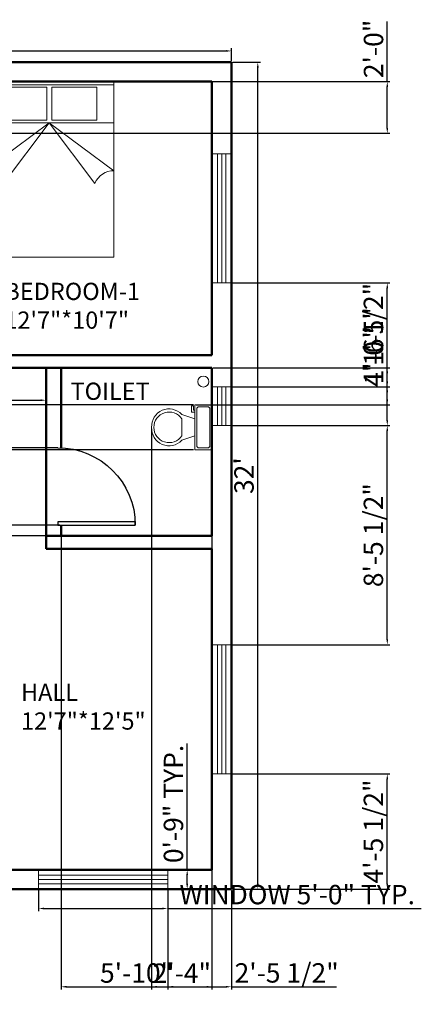
# Model space of a CAD drawing. Units: inches. Extents: x 2181 to 2717, y 1819 to 2296.
# Tile 5 of 5: x 2531 to 2717, y 1819 to 2276. Entities that reach past the tile are written whole.
import ezdxf

# ---------------------------------------------------------------- set-up
doc = ezdxf.new("R2010")
doc.units = ezdxf.units.IN
for name, color, linetype, lineweight in [('A-ANNO-DIMS', 2, 'Continuous', 13), ('A-AREA-IDEN', 7, 'Continuous', 25), ('A-DOOR', 3, 'Continuous', 25), ('A-FLOR-FIXT', 8, 'Continuous', 18), ('A-FURN', 8, 'Continuous', 18), ('A-GLAZ', 4, 'Continuous', 18), ('A-WALL', 7, 'Continuous', 50)]:
    doc.layers.add(name, color=color, linetype=linetype, lineweight=lineweight)
doc.styles.get("Standard").update_dxf_attribs({"font": 'arial.ttf'})
doc.dimstyles.new('ISO-25', dxfattribs={"dimtxt": 9, "dimasz": 2.5, "dimexe": 1.25, "dimexo": 0.625, "dimtad": 1, "dimlunit": 3, "dimtxsty": 'Standard', "dimcen": 2.5, "dimadec": 0, "dimazin": 0, "dimtfac": 1, "dimtmove": 0, "dimatfit": 3, "dimfxl": 1, "dimarcsym": 0})

# ---------------------------------------------------------------- blocks, each defined once
blk = doc.blocks.new('*U4')
for p, q in [((9.5, -6), (9.5, -2)), ((-10, -8.5), (-8, -8.5)), ((-10, -9.5), (-10, -8.5)), ((-8, -8.5), (-8, -8)), ((-7, -8), (-7, -9.5)), ((-4, -8), (-6, -14)), ((4, -8), (6, -14)), ((-7, -9.5), (-10, -9.5)), ((4, -14), (-4, -14))]:
    blk.add_line(p, q)
blk.add_lwpolyline([(10.5, -8), (10.5, 0), (-10.5, 0), (-10.5, -8)], close=True)
for points in [[(-9.5, -2), (-9.5, -6)], [(8.5, -1), (-8.5, -1)], [(-8.5, -7), (8.5, -7)]]:
    blk.add_lwpolyline(points)
for centre, radius, start, end in [((-8.625, -1.875), 0.8839, 81.8699, 188.1301), ((8.625, -1.875), 0.8839, 351.8699, 98.1301), ((-8.625, -6.125), 0.8839, 171.869898, 278.1301), ((8.625, -6.125), 0.8839, 261.8699, 8.1301), ((-0.4772, -19.9188), 8.0953, 133.01722, 273.38), ((0.0374, -19.8731), 7.127, 124.50543, 269.7), ((-0.0373, -19.8731), 7.127, 270.3, 55.4946), ((0.4773, -19.9188), 8.0953, 266.62, 46.9828)]:
    blk.add_arc(centre, radius, start, end)
blk = doc.blocks.new('*U2')
for p, q in [((0, 0), (0, -6)), ((40, 0), (40, -6))]:
    blk.add_line(p, q)
blk.add_lwpolyline([(0, 0), (0, 40), (1.75, 40), (1.75, 0)], close=True)
blk.add_arc((0, 0), 40, 0, 90)
blk = doc.blocks.new('*D8')
at = {"layer": 'A-ANNO-DIMS', "color": 0, "lineweight": -2, "transparency": 16777216}
for p, q in [((2329.35, 2256.83), (2329.35, 2262.67)), ((2331.85, 2261.42), (2626.85, 2261.42)), ((2629.35, 2256.83), (2629.35, 2262.67))]:
    blk.add_line(p, q, dxfattribs=at)
at = {"layer": 'A-ANNO-DIMS', "color": 0, "transparency": 16777216}
for points in [[(2331.85, 2261.84), (2331.85, 2261.01), (2329.35, 2261.42)], [(2626.85, 2261.84), (2626.85, 2261.01), (2629.35, 2261.42)]]:
    blk.add_solid(points, dxfattribs=at)
at = {"layer": 'Defpoints', "color": 0, "transparency": 16777216}
for p in [(2629.35, 2261.42), (2329.35, 2256.2), (2629.35, 2256.2)]:
    blk.add_point(p, dxfattribs=at)
at = {"layer": 'A-ANNO-DIMS', "color": 0, "transparency": 16777216, "insert": (2479.35, 2266.64), "char_height": 9, "attachment_point": 5}
blk.add_mtext("25'", dxfattribs=at)
blk = doc.blocks.new('*D9')
at = {"layer": 'A-ANNO-DIMS', "color": 0, "lineweight": -2, "transparency": 16777216}
for p, q in [((2629.97, 2256.2), (2642.85, 2256.2)), ((2641.6, 1874.7), (2641.6, 2253.7)), ((2629.97, 1872.2), (2642.85, 1872.2))]:
    blk.add_line(p, q, dxfattribs=at)
at = {"layer": 'A-ANNO-DIMS', "color": 0, "transparency": 16777216}
for points in [[(2641.19, 2253.7), (2642.02, 2253.7), (2641.6, 2256.2)], [(2641.19, 1874.7), (2642.02, 1874.7), (2641.6, 1872.2)]]:
    blk.add_solid(points, dxfattribs=at)
at = {"layer": 'Defpoints', "color": 0, "transparency": 16777216}
for p in [(2629.35, 2256.2), (2641.6, 2256.2), (2629.35, 1872.2)]:
    blk.add_point(p, dxfattribs=at)
at = {"layer": 'A-ANNO-DIMS', "color": 0, "transparency": 16777216, "insert": (2636.38, 2064.2), "char_height": 9, "attachment_point": 5, "rotation": 90}
blk.add_mtext("32'", dxfattribs=at)
blk = doc.blocks.new('*D13')
at = {"layer": 'A-ANNO-DIMS', "color": 0, "lineweight": -2, "transparency": 16777216}
for p, q in [((2445.35, 2113.58), (2445.35, 2097.98)), ((2543.35, 2113.58), (2543.35, 2097.98)), ((2447.85, 2099.23), (2540.85, 2099.23))]:
    blk.add_line(p, q, dxfattribs=at)
at = {"layer": 'A-ANNO-DIMS', "color": 0, "transparency": 16777216}
for points in [[(2447.85, 2099.65), (2447.85, 2098.81), (2445.35, 2099.23)], [(2540.85, 2099.65), (2540.85, 2098.81), (2543.35, 2099.23)]]:
    blk.add_solid(points, dxfattribs=at)
at = {"layer": 'Defpoints', "color": 0, "transparency": 16777216}
for p in [(2445.35, 2114.2), (2543.35, 2114.2), (2543.35, 2099.23)]:
    blk.add_point(p, dxfattribs=at)
at = {"layer": 'A-ANNO-DIMS', "color": 0, "transparency": 16777216, "insert": (2494.35, 2104.45), "char_height": 9, "attachment_point": 5}
blk.add_mtext('8\'-2"', dxfattribs=at)
blk = doc.blocks.new('WIN-60IN')
for p, q in [((0, 0), (0, 9)), ((60, 6.5), (0, 6.5)), ((60, 0), (60, 9)), ((60, 4.5), (0, 4.5)), ((60, 2.5), (0, 2.5))]:
    blk.add_line(p, q)
blk = doc.blocks.new('BED-QUEEN-PLAN')
for p, q in [((60.01, 81.47), (0, 81.47)), ((0, 81.47), (0, 80)), ((0.01, 0), (0.01, 80)), ((0.01, 80), (60.01, 80)), ((8.01, 78.8), (28.81, 78.8)), ((8.01, 63.6), (8.01, 78.8)), ((28.81, 78.8), (28.81, 63.6)), ((31.21, 78.8), (52.01, 78.8)), ((31.21, 63.6), (31.21, 78.8)), ((52.01, 78.8), (52.01, 63.6)), ((60.01, 80), (60.01, 81.47)), ((60.01, 80), (60.01, 0)), ((60.01, 62.35), (0.01, 62.35)), ((30.01, 62.35), (0.01, 40)), ((28.81, 63.6), (8.01, 63.6)), ((8.81, 34.19), (30.01, 62.35)), ((30.01, 62.35), (60.01, 40)), ((51.22, 34.19), (30.01, 62.35)), ((52.01, 63.6), (31.21, 63.6)), ((60.01, 0), (0.01, 0))]:
    blk.add_line(p, q)
for centre, start, end in [((0.34, 30.93), 21.0875, 92.0428), ((59.69, 30.93), 87.9572, 158.9125)]:
    blk.add_arc(centre, 9.08, start, end)
blk = doc.blocks.new('*D17')
at = {"layer": 'A-ANNO-DIMS', "color": 0, "lineweight": -2, "transparency": 16777216}
for p, q in [((2539.85, 1871.58), (2539.85, 1861.95)), ((2599.85, 1871.58), (2599.85, 1861.95)), ((2542.35, 1863.2), (2597.35, 1863.2)), ((2599.85, 1863.2), (2717.48, 1863.2))]:
    blk.add_line(p, q, dxfattribs=at)
at = {"layer": 'A-ANNO-DIMS', "color": 0, "transparency": 16777216}
for points in [[(2542.35, 1863.62), (2542.35, 1862.79), (2539.85, 1863.2)], [(2597.35, 1863.62), (2597.35, 1862.79), (2599.85, 1863.2)]]:
    blk.add_solid(points, dxfattribs=at)
at = {"layer": 'Defpoints', "color": 0, "transparency": 16777216}
for p in [(2539.85, 1872.2), (2599.85, 1872.2), (2599.85, 1863.2)]:
    blk.add_point(p, dxfattribs=at)
at = {"layer": 'A-ANNO-DIMS', "color": 0, "transparency": 16777216, "insert": (2659.92, 1868.49), "char_height": 9, "attachment_point": 5}
blk.add_mtext('WINDOW 5\'-0" TYP.', dxfattribs=at)
blk = doc.blocks.new('*D18')
at = {"layer": 'A-ANNO-DIMS', "color": 0, "lineweight": -2, "transparency": 16777216}
for p, q in [((2608.85, 1881.2), (2608.85, 1939.81)), ((2600.47, 1881.2), (2610.1, 1881.2)), ((2608.85, 1874.7), (2608.85, 1878.7)), ((2600.47, 1872.2), (2610.1, 1872.2))]:
    blk.add_line(p, q, dxfattribs=at)
at = {"layer": 'A-ANNO-DIMS', "color": 0, "transparency": 16777216}
for points in [[(2608.43, 1878.7), (2609.26, 1878.7), (2608.85, 1881.2)], [(2608.43, 1874.7), (2609.26, 1874.7), (2608.85, 1872.2)]]:
    blk.add_solid(points, dxfattribs=at)
at = {"layer": 'Defpoints', "color": 0, "transparency": 16777216}
for p in [(2599.85, 1881.2), (2608.85, 1881.2), (2599.85, 1872.2)]:
    blk.add_point(p, dxfattribs=at)
at = {"layer": 'A-ANNO-DIMS', "color": 0, "transparency": 16777216, "insert": (2603.63, 1911.76), "char_height": 9, "attachment_point": 5, "rotation": 90}
blk.add_mtext('0\'-9" TYP.', dxfattribs=at)
blk = doc.blocks.new('*D29')
at = {"layer": 'A-ANNO-DIMS', "color": 0, "lineweight": -2, "transparency": 16777216}
for p, q in [((2701.7, 2105.45), (2701.7, 2132.28)), ((2629.97, 2105.45), (2702.95, 2105.45)), ((2701.7, 2089.95), (2701.7, 2102.95)), ((2629.97, 2087.45), (2702.95, 2087.45))]:
    blk.add_line(p, q, dxfattribs=at)
at = {"layer": 'A-ANNO-DIMS', "color": 0, "transparency": 16777216}
for points in [[(2701.28, 2102.95), (2702.11, 2102.95), (2701.7, 2105.45)], [(2701.28, 2089.95), (2702.11, 2089.95), (2701.7, 2087.45)]]:
    blk.add_solid(points, dxfattribs=at)
at = {"layer": 'Defpoints', "color": 0, "transparency": 16777216}
for p in [(2629.35, 2105.45), (2701.7, 2105.45), (2629.35, 2087.45)]:
    blk.add_point(p, dxfattribs=at)
at = {"layer": 'A-ANNO-DIMS', "color": 0, "transparency": 16777216, "insert": (2696.48, 2120.11), "char_height": 9, "attachment_point": 5, "rotation": 90}
blk.add_mtext('1\'-6"', dxfattribs=at)
blk = doc.blocks.new('*D30')
at = {"layer": 'A-ANNO-DIMS', "color": 0, "lineweight": -2, "transparency": 16777216}
for p, q in [((2629.97, 2087.45), (2702.95, 2087.45)), ((2701.7, 1988.2), (2701.7, 2084.95)), ((2629.97, 1985.7), (2702.95, 1985.7))]:
    blk.add_line(p, q, dxfattribs=at)
at = {"layer": 'A-ANNO-DIMS', "color": 0, "transparency": 16777216}
for points in [[(2701.28, 2084.95), (2702.11, 2084.95), (2701.7, 2087.45)], [(2701.28, 1988.2), (2702.11, 1988.2), (2701.7, 1985.7)]]:
    blk.add_solid(points, dxfattribs=at)
at = {"layer": 'Defpoints', "color": 0, "transparency": 16777216}
for p in [(2629.35, 2087.45), (2701.7, 2087.45), (2629.35, 1985.7)]:
    blk.add_point(p, dxfattribs=at)
at = {"layer": 'A-ANNO-DIMS', "color": 0, "transparency": 16777216, "insert": (2696.42, 2036.58), "char_height": 9, "attachment_point": 5, "rotation": 90}
blk.add_mtext('8\'-5 1/2"', dxfattribs=at)
blk = doc.blocks.new('*D31')
at = {"layer": 'A-ANNO-DIMS', "color": 0, "lineweight": -2, "transparency": 16777216}
for p, q in [((2629.97, 2153.7), (2702.95, 2153.7)), ((2701.7, 2107.95), (2701.7, 2151.2)), ((2629.97, 2105.45), (2702.95, 2105.45))]:
    blk.add_line(p, q, dxfattribs=at)
at = {"layer": 'A-ANNO-DIMS', "color": 0, "transparency": 16777216}
for points in [[(2701.28, 2151.2), (2702.11, 2151.2), (2701.7, 2153.7)], [(2701.28, 2107.95), (2702.11, 2107.95), (2701.7, 2105.45)]]:
    blk.add_solid(points, dxfattribs=at)
at = {"layer": 'Defpoints', "color": 0, "transparency": 16777216}
for p in [(2629.35, 2153.7), (2701.7, 2153.7), (2629.35, 2105.45)]:
    blk.add_point(p, dxfattribs=at)
at = {"layer": 'A-ANNO-DIMS', "color": 0, "transparency": 16777216, "insert": (2696.42, 2129.58), "char_height": 9, "attachment_point": 5, "rotation": 90}
blk.add_mtext('4\'-0 1/2"', dxfattribs=at)
blk = doc.blocks.new('*D32')
at = {"layer": 'A-ANNO-DIMS', "color": 0, "lineweight": -2, "transparency": 16777216}
for p, q in [((2629.97, 1925.7), (2702.95, 1925.7)), ((2701.7, 1874.7), (2701.7, 1923.2)), ((2629.97, 1872.2), (2702.95, 1872.2))]:
    blk.add_line(p, q, dxfattribs=at)
at = {"layer": 'A-ANNO-DIMS', "color": 0, "transparency": 16777216}
for points in [[(2701.28, 1923.2), (2702.11, 1923.2), (2701.7, 1925.7)], [(2701.28, 1874.7), (2702.11, 1874.7), (2701.7, 1872.2)]]:
    blk.add_solid(points, dxfattribs=at)
at = {"layer": 'Defpoints', "color": 0, "transparency": 16777216}
for p in [(2629.35, 1925.7), (2701.7, 1925.7), (2629.35, 1872.2)]:
    blk.add_point(p, dxfattribs=at)
at = {"layer": 'A-ANNO-DIMS', "color": 0, "transparency": 16777216, "insert": (2696.42, 1898.95), "char_height": 9, "attachment_point": 5, "rotation": 90}
blk.add_mtext('4\'-5 1/2"', dxfattribs=at)
blk = doc.blocks.new('*D33')
at = {"layer": 'A-ANNO-DIMS', "color": 0, "lineweight": -2, "transparency": 16777216}
for p, q in [((2599.85, 1871.58), (2599.85, 1825.6)), ((2629.35, 1871.58), (2629.35, 1825.6)), ((2602.35, 1826.85), (2626.85, 1826.85)), ((2629.35, 1826.85), (2678.15, 1826.85))]:
    blk.add_line(p, q, dxfattribs=at)
at = {"layer": 'A-ANNO-DIMS', "color": 0, "transparency": 16777216}
for points in [[(2602.35, 1827.27), (2602.35, 1826.44), (2599.85, 1826.85)], [(2626.85, 1827.27), (2626.85, 1826.44), (2629.35, 1826.85)]]:
    blk.add_solid(points, dxfattribs=at)
at = {"layer": 'Defpoints', "color": 0, "transparency": 16777216}
for p in [(2599.85, 1872.2), (2629.35, 1872.2), (2629.35, 1826.85)]:
    blk.add_point(p, dxfattribs=at)
at = {"layer": 'A-ANNO-DIMS', "color": 0, "transparency": 16777216, "insert": (2655, 1832.13), "char_height": 9, "attachment_point": 5}
blk.add_mtext('2\'-5 1/2"', dxfattribs=at)
blk = doc.blocks.new('*D39')
at = {"layer": 'A-ANNO-DIMS', "color": 0, "lineweight": -2, "transparency": 16777216}
for p, q in [((2550.35, 2035.58), (2550.35, 1825.6)), ((2620.35, 2035.58), (2620.35, 1825.6)), ((2552.85, 1826.85), (2617.85, 1826.85))]:
    blk.add_line(p, q, dxfattribs=at)
at = {"layer": 'A-ANNO-DIMS', "color": 0, "transparency": 16777216}
for points in [[(2552.85, 1827.27), (2552.85, 1826.44), (2550.35, 1826.85)], [(2617.85, 1827.27), (2617.85, 1826.44), (2620.35, 1826.85)]]:
    blk.add_solid(points, dxfattribs=at)
at = {"layer": 'Defpoints', "color": 0, "transparency": 16777216}
for p in [(2550.35, 2036.2), (2620.35, 2036.2), (2620.35, 1826.85)]:
    blk.add_point(p, dxfattribs=at)
at = {"layer": 'A-ANNO-DIMS', "color": 0, "transparency": 16777216, "insert": (2585.35, 1832.07), "char_height": 9, "attachment_point": 5}
blk.add_mtext('5\'-10"', dxfattribs=at)
blk = doc.blocks.new('*D42')
at = {"layer": 'A-ANNO-DIMS', "color": 0, "lineweight": -2, "transparency": 16777216}
for p, q in [((2701.7, 2247.2), (2701.7, 2275.03)), ((2462.97, 2247.2), (2702.95, 2247.2)), ((2701.7, 2225.7), (2701.7, 2244.7)), ((2462.97, 2223.2), (2702.95, 2223.2))]:
    blk.add_line(p, q, dxfattribs=at)
at = {"layer": 'A-ANNO-DIMS', "color": 0, "transparency": 16777216}
for points in [[(2701.28, 2244.7), (2702.11, 2244.7), (2701.7, 2247.2)], [(2701.28, 2225.7), (2702.11, 2225.7), (2701.7, 2223.2)]]:
    blk.add_solid(points, dxfattribs=at)
at = {"layer": 'Defpoints', "color": 0, "transparency": 16777216}
for p in [(2462.35, 2247.2), (2701.7, 2247.2), (2462.35, 2223.2)]:
    blk.add_point(p, dxfattribs=at)
at = {"layer": 'A-ANNO-DIMS', "color": 0, "transparency": 16777216, "insert": (2696.48, 2262.37), "char_height": 9, "attachment_point": 5, "rotation": 90}
blk.add_mtext('2\'-0"', dxfattribs=at)
blk = doc.blocks.new('*D49')
at = {"layer": 'A-ANNO-DIMS', "color": 0, "lineweight": -2, "transparency": 16777216}
for p, q in [((2701.7, 2114.2), (2701.7, 2141.03)), ((2620.97, 2114.2), (2702.95, 2114.2)), ((2701.7, 2099.63), (2701.7, 2111.7)), ((2612.97, 2097.13), (2702.95, 2097.13))]:
    blk.add_line(p, q, dxfattribs=at)
at = {"layer": 'A-ANNO-DIMS', "color": 0, "transparency": 16777216}
for points in [[(2701.28, 2111.7), (2702.11, 2111.7), (2701.7, 2114.2)], [(2701.28, 2099.63), (2702.11, 2099.63), (2701.7, 2097.13)]]:
    blk.add_solid(points, dxfattribs=at)
at = {"layer": 'Defpoints', "color": 0, "transparency": 16777216}
for p in [(2620.35, 2114.2), (2701.7, 2114.2), (2612.35, 2097.13)]:
    blk.add_point(p, dxfattribs=at)
at = {"layer": 'A-ANNO-DIMS', "color": 0, "transparency": 16777216, "insert": (2696.48, 2128.87), "char_height": 9, "attachment_point": 5, "rotation": 90}
blk.add_mtext('1\'-5"', dxfattribs=at)
blk = doc.blocks.new('*D50')
at = {"layer": 'A-ANNO-DIMS', "color": 0, "lineweight": -2, "transparency": 16777216}
for p, q in [((2308, 2097.13), (2308, 2123.96)), ((2611.72, 2097.13), (2306.75, 2097.13)), ((2308, 2078.63), (2308, 2094.63)), ((2611.72, 2076.13), (2306.75, 2076.13))]:
    blk.add_line(p, q, dxfattribs=at)
at = {"layer": 'A-ANNO-DIMS', "color": 0, "transparency": 16777216}
for points in [[(2307.58, 2094.63), (2308.41, 2094.63), (2308, 2097.13)], [(2307.58, 2078.63), (2308.41, 2078.63), (2308, 2076.13)]]:
    blk.add_solid(points, dxfattribs=at)
at = {"layer": 'Defpoints', "color": 0, "transparency": 16777216}
for p in [(2308, 2097.13), (2612.35, 2097.13), (2612.35, 2076.13)]:
    blk.add_point(p, dxfattribs=at)
at = {"layer": 'A-ANNO-DIMS', "color": 0, "transparency": 16777216, "insert": (2302.78, 2111.79), "char_height": 9, "attachment_point": 5, "rotation": 90}
blk.add_mtext('1\'-9"', dxfattribs=at)
blk = doc.blocks.new('*D51')
at = {"layer": 'A-ANNO-DIMS', "color": 0, "lineweight": -2, "transparency": 16777216}
for p, q in [((2592.35, 2086), (2592.35, 1825.6)), ((2620.35, 2075.5), (2620.35, 1825.6)), ((2594.85, 1826.85), (2617.85, 1826.85))]:
    blk.add_line(p, q, dxfattribs=at)
at = {"layer": 'A-ANNO-DIMS', "color": 0, "transparency": 16777216}
for points in [[(2594.85, 1827.27), (2594.85, 1826.44), (2592.35, 1826.85)], [(2617.85, 1827.27), (2617.85, 1826.44), (2620.35, 1826.85)]]:
    blk.add_solid(points, dxfattribs=at)
at = {"layer": 'Defpoints', "color": 0, "transparency": 16777216}
for p in [(2592.35, 2086.63), (2620.35, 2076.13), (2620.35, 1826.85)]:
    blk.add_point(p, dxfattribs=at)
at = {"layer": 'A-ANNO-DIMS', "color": 0, "transparency": 16777216, "insert": (2606.35, 1832), "char_height": 9, "attachment_point": 5}
blk.add_mtext('2\'-4"', dxfattribs=at)
blk = doc.blocks.new('*D52')
at = {"layer": 'A-ANNO-DIMS', "color": 0, "lineweight": -2, "transparency": 16777216}
for p, q in [((2542.72, 2077.19), (2306.75, 2077.19)), ((2308, 2043.69), (2308, 2074.69)), ((2542.72, 2041.19), (2306.75, 2041.19))]:
    blk.add_line(p, q, dxfattribs=at)
at = {"layer": 'A-ANNO-DIMS', "color": 0, "transparency": 16777216}
for points in [[(2307.58, 2074.69), (2308.41, 2074.69), (2308, 2077.19)], [(2307.58, 2043.69), (2308.41, 2043.69), (2308, 2041.19)]]:
    blk.add_solid(points, dxfattribs=at)
at = {"layer": 'Defpoints', "color": 0, "transparency": 16777216}
for p in [(2308, 2077.19), (2543.35, 2077.19), (2543.35, 2041.19)]:
    blk.add_point(p, dxfattribs=at)
at = {"layer": 'A-ANNO-DIMS', "color": 0, "transparency": 16777216, "insert": (2302.77, 2059.19), "char_height": 9, "attachment_point": 5, "rotation": 90}
blk.add_mtext('3\'-0"', dxfattribs=at)
blk = doc.blocks.new('*D53')
at = {"layer": 'A-ANNO-DIMS', "color": 0, "lineweight": -2, "transparency": 16777216}
for p, q in [((2308, 2043.69), (2308, 2046.19)), ((2549.72, 2041.19), (2306.75, 2041.19)), ((2308, 2041.19), (2308, 2036.2)), ((2549.72, 2036.2), (2306.75, 2036.2)), ((2308, 2033.7), (2308, 2006.03))]:
    blk.add_line(p, q, dxfattribs=at)
at = {"layer": 'A-ANNO-DIMS', "color": 0, "transparency": 16777216}
for points in [[(2307.58, 2043.69), (2308.41, 2043.69), (2308, 2041.19)], [(2307.58, 2033.7), (2308.41, 2033.7), (2308, 2036.2)]]:
    blk.add_solid(points, dxfattribs=at)
at = {"layer": 'Defpoints', "color": 0, "transparency": 16777216}
for p in [(2550.35, 2041.19), (2308, 2036.2), (2550.35, 2036.2)]:
    blk.add_point(p, dxfattribs=at)
at = {"layer": 'A-ANNO-DIMS', "color": 0, "transparency": 16777216, "insert": (2302.78, 2018.62), "char_height": 9, "attachment_point": 5, "rotation": 90}
blk.add_mtext('0\'-5"', dxfattribs=at)
blk = doc.blocks.new('*D56')
at = {"layer": 'A-ANNO-DIMS', "color": 0, "lineweight": -2, "transparency": 16777216}
for p, q in [((2549.72, 2114.2), (2306.75, 2114.2)), ((2308, 2038.7), (2308, 2111.7)), ((2549.72, 2036.2), (2306.75, 2036.2))]:
    blk.add_line(p, q, dxfattribs=at)
at = {"layer": 'A-ANNO-DIMS', "color": 0, "transparency": 16777216}
for points in [[(2307.58, 2111.7), (2308.41, 2111.7), (2308, 2114.2)], [(2307.58, 2038.7), (2308.41, 2038.7), (2308, 2036.2)]]:
    blk.add_solid(points, dxfattribs=at)
at = {"layer": 'Defpoints', "color": 0, "transparency": 16777216}
for p in [(2308, 2114.2), (2550.35, 2114.2), (2550.35, 2036.2)]:
    blk.add_point(p, dxfattribs=at)
at = {"layer": 'A-ANNO-DIMS', "color": 0, "transparency": 16777216, "insert": (2302.78, 2075.2), "char_height": 9, "attachment_point": 5, "rotation": 90}
blk.add_mtext('6\'-6"', dxfattribs=at)

msp = doc.modelspace()

# ---------------------------------------------------------------- linework, layer by layer
at = {"layer": 'A-FLOR-FIXT'}
msp.add_circle((2616.346, 2107.897), 2.575, dxfattribs=at)
at = {"layer": 'A-GLAZ'}
for p, q in [((2620.346, 2105.45), (2629.346, 2105.45)), ((2622.846, 2105.45), (2622.846, 2087.45)), ((2624.846, 2105.45), (2624.846, 2087.45)), ((2626.846, 2105.45), (2626.846, 2087.45)), ((2620.346, 2087.45), (2629.346, 2087.45))]:
    msp.add_line(p, q, dxfattribs=at)
at = {"layer": 'A-WALL'}
for p, q in [((2329.346, 2256.205), (2629.346, 2256.205)), ((2629.346, 2256.205), (2629.346, 1872.205)), ((2469.346, 2247.205), (2620.346, 2247.205)), ((2620.346, 2247.205), (2620.346, 2120.205)), ((2510.745, 2120.205), (2620.346, 2120.205)), ((2338.346, 2114.205), (2620.346, 2114.205)), ((2543.346, 2114.205), (2543.346, 2030.205)), ((2550.346, 2114.205), (2550.346, 2077.152)), ((2620.346, 2114.205), (2620.346, 2036.205)), ((2550.346, 2041.187), (2550.346, 2036.205)), ((2543.346, 2036.205), (2620.346, 2036.205)), ((2543.346, 2030.205), (2620.346, 2030.205)), ((2620.346, 2030.205), (2620.346, 1881.205)), ((2519.346, 1881.205), (2620.346, 1881.205)), ((2329.346, 1872.205), (2629.346, 1872.205))]:
    msp.add_line(p, q, dxfattribs=at)

# ---------------------------------------------------------------- block references
at = {"layer": 'A-DOOR', "xscale": -0.9, "yscale": 0.9, "zscale": 0.9, "rotation": 270}
msp.add_blockref('*U2', (2548.746, 2041.187), dxfattribs=at)
at = {"layer": 'A-FLOR-FIXT', "rotation": 270.0000000000003}
msp.add_blockref('*U4', (2620.346, 2086.628), dxfattribs=at)
at = {"layer": 'A-FURN'}
msp.add_blockref('BED-QUEEN-PLAN', (2514.834, 2165.732), dxfattribs=at)
at = {"layer": 'A-GLAZ'}
for p, rotation in [((2620.347, 2213.705), 270.0000000000003), ((2620.347, 1985.705), 269.9999999999999)]:
    msp.add_blockref('WIN-60IN', p, dxfattribs=dict(at, rotation=rotation))
msp.add_blockref('WIN-60IN', (2539.846, 1872.205), dxfattribs=at)

# ---------------------------------------------------------------- texts
at = {"layer": 'A-AREA-IDEN', "char_height": 8, "attachment_point": 1}
for s, width, insert in [('BEDROOM-1\\P12\'7"*10\'7"', 37.99236, (2523.994, 2153.766)), ('TOILET', 27.2831, (2554.717, 2107.388)), ('HALL\\P12\'7"*12\'5"', 52.01638, (2531.721, 1967.594))]:
    msp.add_mtext_dynamic_manual_height_columns(s, width=width, gutter_width=12.5, heights=[0], dxfattribs=dict(at, insert=insert))

# ---------------------------------------------------------------- dimensions: what is measured, and where the dimension line sits
at = {"layer": 'A-ANNO-DIMS'}
dim = msp.add_linear_dim(base=(2629.346, 2261.425), p1=(2329.346, 2256.205), p2=(2629.346, 2256.205), dimstyle='ISO-25', override={"dimclrd": 0, "dimclre": 0, "dimclrt": 0}, dxfattribs=at)
dim.commit()
dim.dimension.update_dxf_attribs({"geometry": '*D8', "text_midpoint": (2479.346, 2261.425), "dimtype": 160})
for base, p1, p2, override, picture, middle in [((2701.696, 2247.205), (2462.346, 2223.205), (2462.346, 2247.205), {"dimdec": 1, "dimlfac": 1, "dimrnd": 0, "dimzin": 1, "dimdsep": 46, "dimlunit": 4, "dimfrac": 2}, '*D42', (2696.476, 2262.368)), ((2641.604, 2256.205), (2629.346, 1872.205), (2629.346, 2256.205), {"dimclrd": 0, "dimclre": 0, "dimclrt": 0}, '*D9', (2636.381, 2064.205)), ((2701.696, 2153.705), (2629.346, 2105.45), (2629.346, 2153.705), {"dimdec": 1, "dimlfac": 1, "dimrnd": 0, "dimzin": 1, "dimdsep": 46, "dimlunit": 4, "dimfrac": 2}, '*D31', (2696.418, 2129.577)), ((2701.696, 2114.205), (2612.346, 2097.128), (2620.346, 2114.205), {"dimdec": 1, "dimlfac": 1, "dimrnd": 0, "dimzin": 1, "dimdsep": 46, "dimlunit": 4, "dimfrac": 2}, '*D49', (2696.476, 2128.868)), ((2701.696, 2105.45), (2629.346, 2087.45), (2629.346, 2105.45), {"dimdec": 1, "dimlfac": 1, "dimrnd": 0, "dimzin": 1, "dimdsep": 46, "dimlunit": 4, "dimfrac": 2}, '*D29', (2696.476, 2120.113)), ((2307.996, 2097.128), (2612.346, 2076.128), (2612.346, 2097.128), {"dimdec": 1, "dimlfac": 1, "dimrnd": 0, "dimzin": 1, "dimdsep": 46, "dimlunit": 4, "dimfrac": 2}, '*D50', (2302.776, 2111.792)), ((2307.996, 2114.205), (2550.346, 2036.205), (2550.346, 2114.205), {"dimdec": 1, "dimlfac": 1, "dimrnd": 0, "dimzin": 1, "dimdsep": 46, "dimlunit": 4, "dimfrac": 2}, '*D56', (2302.776, 2075.205)), ((2701.696, 2087.45), (2629.346, 1985.705), (2629.346, 2087.45), {"dimdec": 1, "dimlfac": 1, "dimrnd": 0, "dimzin": 1, "dimdsep": 46, "dimlunit": 4, "dimfrac": 2}, '*D30', (2696.418, 2036.577)), ((2307.996, 2077.187), (2543.346, 2041.187), (2543.346, 2077.187), {"dimdec": 1, "dimlfac": 1, "dimrnd": 0, "dimzin": 1, "dimdsep": 46, "dimlunit": 4, "dimfrac": 2}, '*D52', (2302.773, 2059.187)), ((2307.996, 2036.205), (2550.346, 2041.187), (2550.346, 2036.205), {"dimdec": 1, "dimlfac": 1, "dimrnd": 0, "dimzin": 1, "dimdsep": 46, "dimlunit": 4, "dimfrac": 2}, '*D53', (2302.776, 2018.617)), ((2701.696, 1925.705), (2629.346, 1872.205), (2629.346, 1925.705), {"dimdec": 1, "dimlfac": 1, "dimrnd": 0, "dimzin": 1, "dimdsep": 46, "dimlunit": 4, "dimfrac": 2}, '*D32', (2696.418, 1898.955))]:
    dim = msp.add_linear_dim(base=base, p1=p1, p2=p2, angle=90, dimstyle='ISO-25', override=override, dxfattribs=at)
    dim.commit()
    dim.dimension.update_dxf_attribs({"geometry": picture, "text_midpoint": middle})
for base, p1, p2, override, picture, middle in [((2543.346, 2099.229), (2445.346, 2114.205), (2543.346, 2114.205), {"dimclrd": 0, "dimclre": 0, "dimclrt": 0}, '*D13', (2494.346, 2104.449)), ((2620.346, 1826.855), (2592.346, 2086.628), (2620.346, 2076.128), {"dimdec": 1, "dimlfac": 1, "dimrnd": 0, "dimzin": 1, "dimdsep": 46, "dimlunit": 4, "dimfrac": 2}, '*D51', (2606.346, 1831.998)), ((2620.346, 1826.855), (2550.346, 2036.205), (2620.346, 2036.205), {"dimdec": 1, "dimlfac": 1, "dimrnd": 0, "dimzin": 1, "dimdsep": 46, "dimlunit": 4, "dimfrac": 2}, '*D39', (2585.346, 1832.075)), ((2629.346, 1826.855), (2599.846, 1872.205), (2629.346, 1872.205), {"dimdec": 1, "dimlfac": 1, "dimrnd": 0, "dimzin": 1, "dimdsep": 46, "dimlunit": 4, "dimfrac": 2}, '*D33', (2654.996, 1832.133))]:
    dim = msp.add_linear_dim(base=base, p1=p1, p2=p2, dimstyle='ISO-25', override=override, dxfattribs=at)
    dim.commit()
    dim.dimension.update_dxf_attribs({"geometry": picture, "text_midpoint": middle})
dim = msp.add_linear_dim(base=(2608.846, 1881.205), p1=(2599.846, 1872.205), p2=(2599.846, 1881.205), angle=90, text='<> TYP.', dimstyle='ISO-25', override={"dimdec": 1, "dimlfac": 1, "dimrnd": 0, "dimzin": 1, "dimdsep": 46, "dimlunit": 4, "dimfrac": 2}, dxfattribs=at)
dim.commit()
dim.dimension.update_dxf_attribs({"geometry": '*D18', "text_midpoint": (2603.626, 1911.759)})
dim = msp.add_linear_dim(base=(2599.846, 1863.205), p1=(2539.846, 1872.205), p2=(2599.846, 1872.205), text='WINDOW <> TYP.', dimstyle='ISO-25', override={"dimdec": 1, "dimlfac": 1, "dimrnd": 0, "dimzin": 1, "dimdsep": 46, "dimlunit": 4, "dimfrac": 2}, dxfattribs=at)
dim.commit()
dim.dimension.update_dxf_attribs({"geometry": '*D17', "text_midpoint": (2659.915, 1868.486)})

doc.saveas('drawing.dxf')
